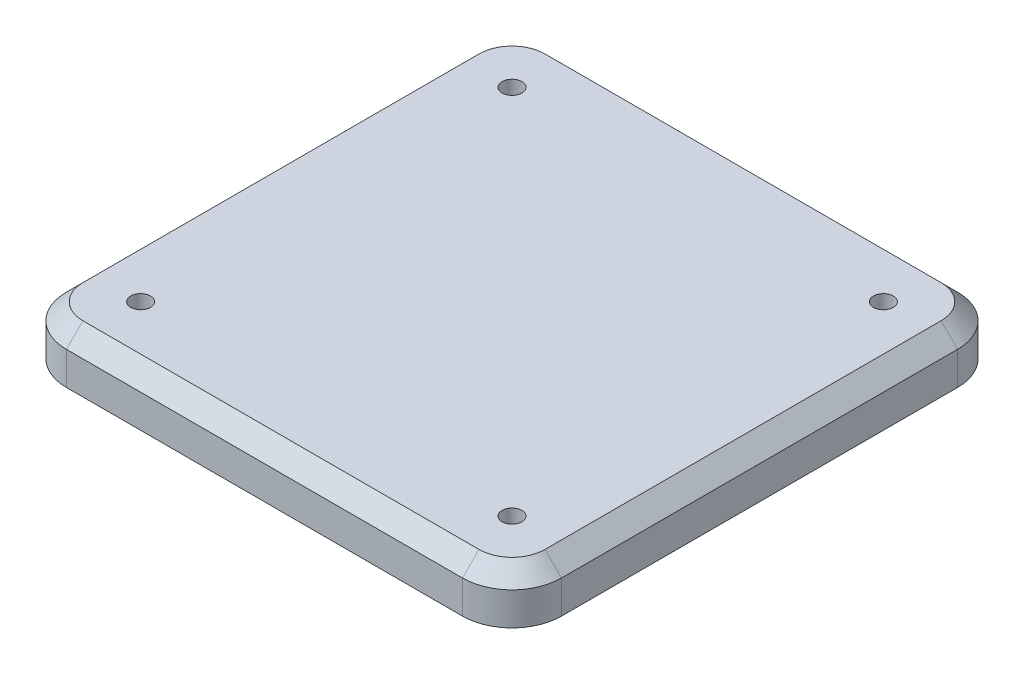
from build123d import *

# Parameters (mm, degrees)
BASE_PLATE_PROFILE_300X300_W       = 300
BASE_PLATE_PROFILE_300X300_H       = 300
BASE_PLATE_300X300X30_DEPTH        = 15
CORNER_FILLETS_R30_R               = 30
EDGE_CHAMFER_10X45_SIZE            = 10
DOWEL_HOLES_12_ON_225_SQUARE_D     = 12
DOWEL_HOLES_12_ON_225_SQUARE_DEPTH = 10
DOWEL_HOLES_12_ON_225_SQUARE_TIP   = 3.605163714
DOWEL_HOLES_12_ON_250_SQUARE_D     = 12
DOWEL_HOLES_12_ON_250_SQUARE_DEPTH = 10
DOWEL_HOLES_12_ON_250_SQUARE_TIP   = 3.605163714


with BuildPart() as part:
    # Base Plate Profile 300x300 → Base Plate 300x300x30 (new, symmetric)
    with BuildSketch(Plane(origin=(0, 0, 0), x_dir=(1, 0, 0), z_dir=(0, 1, 0))):
        Rectangle(BASE_PLATE_PROFILE_300X300_W, BASE_PLATE_PROFILE_300X300_H)
    extrude(amount=BASE_PLATE_300X300X30_DEPTH, both=True)

    # Corner Fillets R30
    corner_fillets_r30_edges = [part.edges().sort_by_distance(p)[0] for p in [
        (150, 0, 150),
        (-150, 0, 150),
        (-150, 0, -150),
        (150, 0, -150),
    ]]
    fillet(corner_fillets_r30_edges, radius=CORNER_FILLETS_R30_R)

    # Edge Chamfer 10x45
    edge_chamfer_10x45_edges = [part.edges().sort_by_distance(p)[0] for p in [
        (0, 15, 150),
        (-150, 15, 0),
        (150, 15, 0),
        (0, 15, -150),
        (141.213203436, 15, -141.213203436),
        (-141.213203436, 15, -141.213203436),
        (141.213203436, 15, 141.213203436),
        (-141.213203436, 15, 141.213203436),
    ]]
    chamfer(edge_chamfer_10x45_edges, length=EDGE_CHAMFER_10X45_SIZE)

    # Dowel Holes Ø12 on 225 Square
    with Locations(Plane(origin=(112.5, 15, -112.5), x_dir=(0, 0, 1), z_dir=(0, 1, 0))):
        with Locations((0, 0), (0, -225), (225, -225), (225, 0)):
            Hole(DOWEL_HOLES_12_ON_225_SQUARE_D / 2, depth=DOWEL_HOLES_12_ON_225_SQUARE_DEPTH)
            with Locations((0, 0, -(DOWEL_HOLES_12_ON_225_SQUARE_DEPTH + DOWEL_HOLES_12_ON_225_SQUARE_TIP / 2))):  # 118° drill point
                Cone(0, DOWEL_HOLES_12_ON_225_SQUARE_D / 2, DOWEL_HOLES_12_ON_225_SQUARE_TIP, mode=Mode.SUBTRACT)

    # Dowel Holes Ø12 on 250 Square
    with Locations(Plane(origin=(-125, -15, 125), x_dir=(0, 0, -1), z_dir=(0, -1, 0))):
        with Locations((0, 0), (0, 250), (250, 250), (250, 0)):
            Hole(DOWEL_HOLES_12_ON_250_SQUARE_D / 2, depth=DOWEL_HOLES_12_ON_250_SQUARE_DEPTH)
            with Locations((0, 0, -(DOWEL_HOLES_12_ON_250_SQUARE_DEPTH + DOWEL_HOLES_12_ON_250_SQUARE_TIP / 2))):  # 118° drill point
                Cone(0, DOWEL_HOLES_12_ON_250_SQUARE_D / 2, DOWEL_HOLES_12_ON_250_SQUARE_TIP, mode=Mode.SUBTRACT)


solid = part.part
